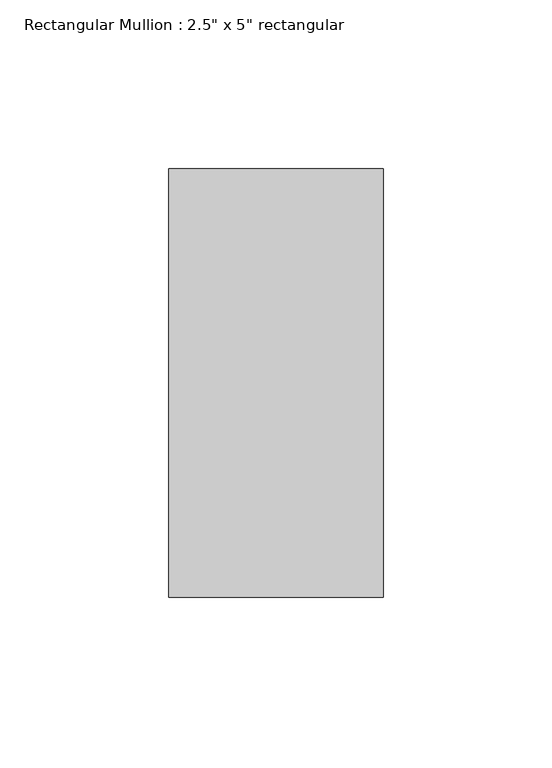
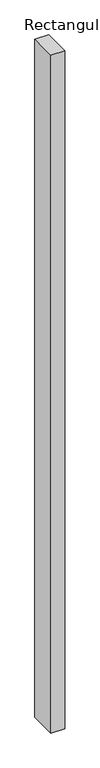
"""IFC4 building model written with IfcOpenShell, lengths in millimetres: member geometry."""

from ifc_helpers import new_model, si_unit, frame, origin, place, context, project, spatial, polyline, outline, extrude, source, transform, mapped, element, save


def member_128fbec0(model_context):
    return source(origin(), model_context, "Body", "SweptSolid", [
        extrude(outline(polyline([(0.0, 63.5), (0.0, -63.5), (-63.5, -63.5), (-63.5, 63.5), (0.0, 63.5)])), frame((0.0, 0.0, -3286.0765121), z_axis=(0.0, 0.0, 1.0), x_axis=(1.0, 0.0, 0.0)), (0.0, 0.0, 1.0), 3286.0765121),
    ])


if __name__ == "__main__":
    model = new_model("IFC4")
    model_context = context("Model", 3, world=origin())
    ifc_project = project(units=[si_unit("LENGTHUNIT", "METRE", prefix="MILLI")], contexts=[model_context])
    site = spatial("IfcSite", under=ifc_project)
    building = spatial("IfcBuilding", under=site)
    placement = place(None, origin())
    member_shape = member_128fbec0(model_context)
    element("IfcMember", 1, ObjectType="Rectangular Mullion : 2.5\" x 5\" rectangular", at=placement, inside=building, context=model_context, shape_type="MappedRepresentation", body=[
        mapped(member_shape, transform((0.0, 0.0, 0.0), x_axis=(1.0, 0.0, 0.0), y_axis=(0.0, 1.0, 0.0), z_axis=(0.0, 0.0, 1.0))),
    ])
    save(model, "model.ifc")

# Revit data of these elements
# Type "Rectangular Mullion : 2.5\" x 5\" rectangular"
#   built-in parameter 1007304 = 0.416667 (stored number, unit not read)
#   built-in parameter 1007301 = 0.104167 (stored number, unit not read)
#   built-in parameter 1007300 = 0.104167 (stored number, unit not read)
# Element 1 (IfcMember, "Rectangular Mullion : 2.5\" x 5\" rectangular")
#   Materials on its faces: "Aluminum"
# Materials
#   "Aluminum": class "Metal", colour RGB 247 247 247, transparency 0, Description = "Aluminum 6061", Cost = 0
